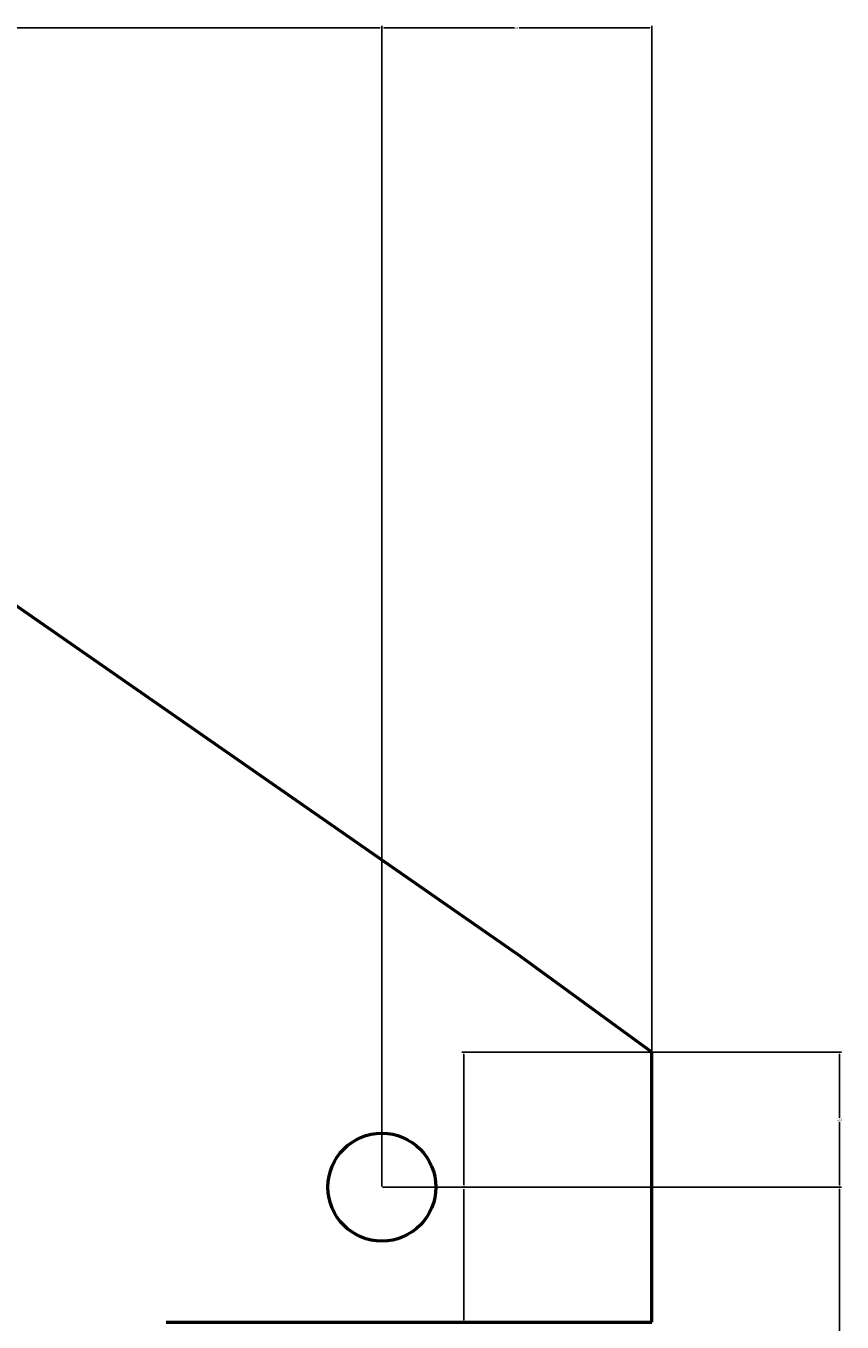
# Model space of a CAD drawing. Units: inches. Extents: x 457 to 775, y 319 to 541.
# Tile 12 of 12: x 699 to 775, y 421 to 541. Entities that reach past the tile are written whole.
import ezdxf

# ---------------------------------------------------------------- set-up
doc = ezdxf.new("R2010")
doc.units = ezdxf.units.IN
doc.header["$MEASUREMENT"] = 0
doc.layers.add('M-DIMS', color=2, linetype='Continuous', lineweight=18)
doc.layers.add('M-OUTL', color=7, linetype='Continuous', lineweight=50)
doc.styles.get("Standard").update_dxf_attribs({"font": 'arial.ttf'})
doc.dimstyles.get("Standard").update_dxf_attribs({"dimtxt": 0.18, "dimasz": 0.18, "dimexe": 0.18, "dimexo": 0.0625, "dimgap": 0.09, "dimtad": 0, "dimtih": 1, "dimtoh": 1, "dimdec": 4, "dimzin": 0, "dimdsep": 46, "dimtxsty": 'Standard', "dimcen": 0.09, "dimadec": 0, "dimazin": 0, "dimtfac": 1, "dimtdec": 4, "dimtofl": 0, "dimtmove": 0, "dimatfit": 3, "dimfxl": 1, "dimtolj": 1, "dimtzin": 0, "dimarcsym": 0})

# ---------------------------------------------------------------- blocks, each defined once
blk = doc.blocks.new('MOUNT-HOLE-D10')
blk.add_circle((5, 5), 5)
blk = doc.blocks.new('*D4')
at = {"layer": 'Defpoints', "color": 0, "transparency": 16777216}
for p in [(731.93, 540.61), (646, 523.21), (731.93, 433.2)]:
    blk.add_point(p, dxfattribs=at)
at = {"layer": 'M-DIMS', "color": 0, "lineweight": -2, "transparency": 16777216}
for p, q in [((646, 523.28), (646, 540.79)), ((646.18, 540.61), (688.57, 540.61)), ((731.75, 540.61), (689.36, 540.61)), ((731.93, 433.26), (731.93, 540.79))]:
    blk.add_line(p, q, dxfattribs=at)
at = {"layer": 'M-DIMS', "color": 0, "transparency": 16777216}
for points in [[(646.18, 540.64), (646.18, 540.58), (646, 540.61)], [(731.75, 540.64), (731.75, 540.58), (731.93, 540.61)]]:
    blk.add_solid(points, dxfattribs=at)
at = {"layer": 'M-DIMS', "color": 0, "transparency": 16777216, "insert": (688.97, 540.61), "char_height": 0.18, "attachment_point": 5}
blk.add_mtext('\\A1;85.93', dxfattribs=at)
blk = doc.blocks.new('*D10')
at = {"layer": 'Defpoints', "color": 0, "transparency": 16777216}
for p in [(756.93, 445.7), (731.93, 433.2), (774.33, 433.2)]:
    blk.add_point(p, dxfattribs=at)
at = {"layer": 'M-DIMS', "color": 0, "lineweight": -2, "transparency": 16777216}
for p, q in [((756.99, 445.7), (774.51, 445.7)), ((774.33, 445.52), (774.33, 439.63)), ((774.33, 433.38), (774.33, 439.26)), ((731.99, 433.2), (774.51, 433.2))]:
    blk.add_line(p, q, dxfattribs=at)
at = {"layer": 'M-DIMS', "color": 0, "transparency": 16777216}
for points in [[(774.3, 445.52), (774.36, 445.52), (774.33, 445.7)], [(774.3, 433.38), (774.36, 433.38), (774.33, 433.2)]]:
    blk.add_solid(points, dxfattribs=at)
at = {"layer": 'M-DIMS', "color": 0, "transparency": 16777216, "insert": (774.33, 439.45), "char_height": 0.18, "attachment_point": 5}
blk.add_mtext('\\A1;12.5', dxfattribs=at)
blk = doc.blocks.new('*D11')
at = {"layer": 'Defpoints', "color": 0, "transparency": 16777216}
for p in [(739.53, 445.7), (756.93, 445.7), (756.93, 420.7)]:
    blk.add_point(p, dxfattribs=at)
at = {"layer": 'M-DIMS', "color": 0, "lineweight": -2, "transparency": 16777216}
for p, q in [((756.87, 445.7), (739.35, 445.7)), ((739.53, 445.52), (739.53, 433.38)), ((739.53, 420.88), (739.53, 433.01)), ((756.87, 420.7), (739.35, 420.7))]:
    blk.add_line(p, q, dxfattribs=at)
at = {"layer": 'M-DIMS', "color": 0, "transparency": 16777216}
for points in [[(739.5, 445.52), (739.56, 445.52), (739.53, 445.7)], [(739.5, 420.88), (739.56, 420.88), (739.53, 420.7)]]:
    blk.add_solid(points, dxfattribs=at)
at = {"layer": 'M-DIMS', "color": 0, "transparency": 16777216, "insert": (739.53, 433.2), "char_height": 0.18, "attachment_point": 5}
blk.add_mtext('\\A1;25', dxfattribs=at)
blk = doc.blocks.new('*D13')
at = {"layer": 'Defpoints', "color": 0, "transparency": 16777216}
for p in [(756.93, 540.61), (756.93, 445.7), (731.93, 433.2)]:
    blk.add_point(p, dxfattribs=at)
at = {"layer": 'M-DIMS', "color": 0, "lineweight": -2, "transparency": 16777216}
for p, q in [((731.93, 433.26), (731.93, 540.79)), ((732.11, 540.61), (744.21, 540.61)), ((756.75, 540.61), (744.65, 540.61)), ((756.93, 445.76), (756.93, 540.79))]:
    blk.add_line(p, q, dxfattribs=at)
at = {"layer": 'M-DIMS', "color": 0, "transparency": 16777216}
for points in [[(732.11, 540.64), (732.11, 540.58), (731.93, 540.61)], [(756.75, 540.64), (756.75, 540.58), (756.93, 540.61)]]:
    blk.add_solid(points, dxfattribs=at)
at = {"layer": 'M-DIMS', "color": 0, "transparency": 16777216, "insert": (744.43, 540.61), "char_height": 0.18, "attachment_point": 5}
blk.add_mtext('\\A1;25', dxfattribs=at)
blk = doc.blocks.new('*D14')
at = {"layer": 'Defpoints', "color": 0, "transparency": 16777216}
for p in [(731.93, 433.2), (774.33, 433.2), (731.93, 388.2)]:
    blk.add_point(p, dxfattribs=at)
at = {"layer": 'M-DIMS', "color": 0, "lineweight": -2, "transparency": 16777216}
for p, q in [((731.99, 433.2), (774.51, 433.2)), ((774.33, 433.02), (774.33, 410.88)), ((774.33, 388.38), (774.33, 410.51)), ((731.99, 388.2), (774.51, 388.2))]:
    blk.add_line(p, q, dxfattribs=at)
at = {"layer": 'M-DIMS', "color": 0, "transparency": 16777216}
for points in [[(774.3, 433.02), (774.36, 433.02), (774.33, 433.2)], [(774.3, 388.38), (774.36, 388.38), (774.33, 388.2)]]:
    blk.add_solid(points, dxfattribs=at)
at = {"layer": 'M-DIMS', "color": 0, "transparency": 16777216, "insert": (774.33, 410.7), "char_height": 0.18, "attachment_point": 5}
blk.add_mtext('\\A1;45', dxfattribs=at)

msp = doc.modelspace()

# ---------------------------------------------------------------- linework, layer by layer
at = {"layer": 'M-OUTL'}
for p, q in [((646.001, 523.213), (744.409, 454.859)), ((756.931, 445.696), (744.409, 454.859)), ((756.931, 420.696), (756.931, 445.696)), ((711.931, 420.696), (756.931, 420.696))]:
    msp.add_line(p, q, dxfattribs=at)

# ---------------------------------------------------------------- block references
msp.add_blockref('MOUNT-HOLE-D10', (726.931, 428.196), dxfattribs=at)

# ---------------------------------------------------------------- dimensions: what is measured, and where the dimension line sits
at = {"layer": 'M-DIMS'}
for base, p1, p2, override, picture, middle in [((731.931, 540.613), (646.001, 523.213), (731.931, 433.196), {"dimdec": 2, "dimlfac": 1, "dimrnd": 0, "dimzin": 0, "dimdsep": 46, "dimlunit": 2}, '*D4', (688.966, 540.613)), ((756.931, 540.613), (731.931, 433.196), (756.931, 445.696), {"dimdec": 0, "dimlfac": 1, "dimrnd": 0, "dimzin": 0, "dimdsep": 46, "dimlunit": 2}, '*D13', (744.431, 540.613))]:
    dim = msp.add_linear_dim(base=base, p1=p1, p2=p2, dimstyle='Standard', override=override, dxfattribs=at)
    dim.commit()
    dim.dimension.update_dxf_attribs({"geometry": picture, "text_midpoint": middle})
for base, p1, p2, override, picture, middle in [((774.331, 433.196), (756.931, 445.696), (731.931, 433.196), {"dimdec": 1, "dimlfac": 1, "dimrnd": 0, "dimzin": 0, "dimdsep": 46, "dimlunit": 2}, '*D10', (774.331, 439.446)), ((739.531, 445.696), (756.931, 420.696), (756.931, 445.696), {"dimdec": 0, "dimlfac": 1, "dimrnd": 0, "dimzin": 0, "dimdsep": 46, "dimlunit": 2}, '*D11', (739.531, 433.196)), ((774.331, 433.196), (731.931, 388.196), (731.931, 433.196), {"dimdec": 0, "dimlfac": 1, "dimrnd": 0, "dimzin": 0, "dimdsep": 46, "dimlunit": 2}, '*D14', (774.331, 410.696))]:
    dim = msp.add_linear_dim(base=base, p1=p1, p2=p2, angle=90, dimstyle='Standard', override=override, dxfattribs=at)
    dim.commit()
    dim.dimension.update_dxf_attribs({"geometry": picture, "text_midpoint": middle})

doc.saveas('drawing.dxf')
